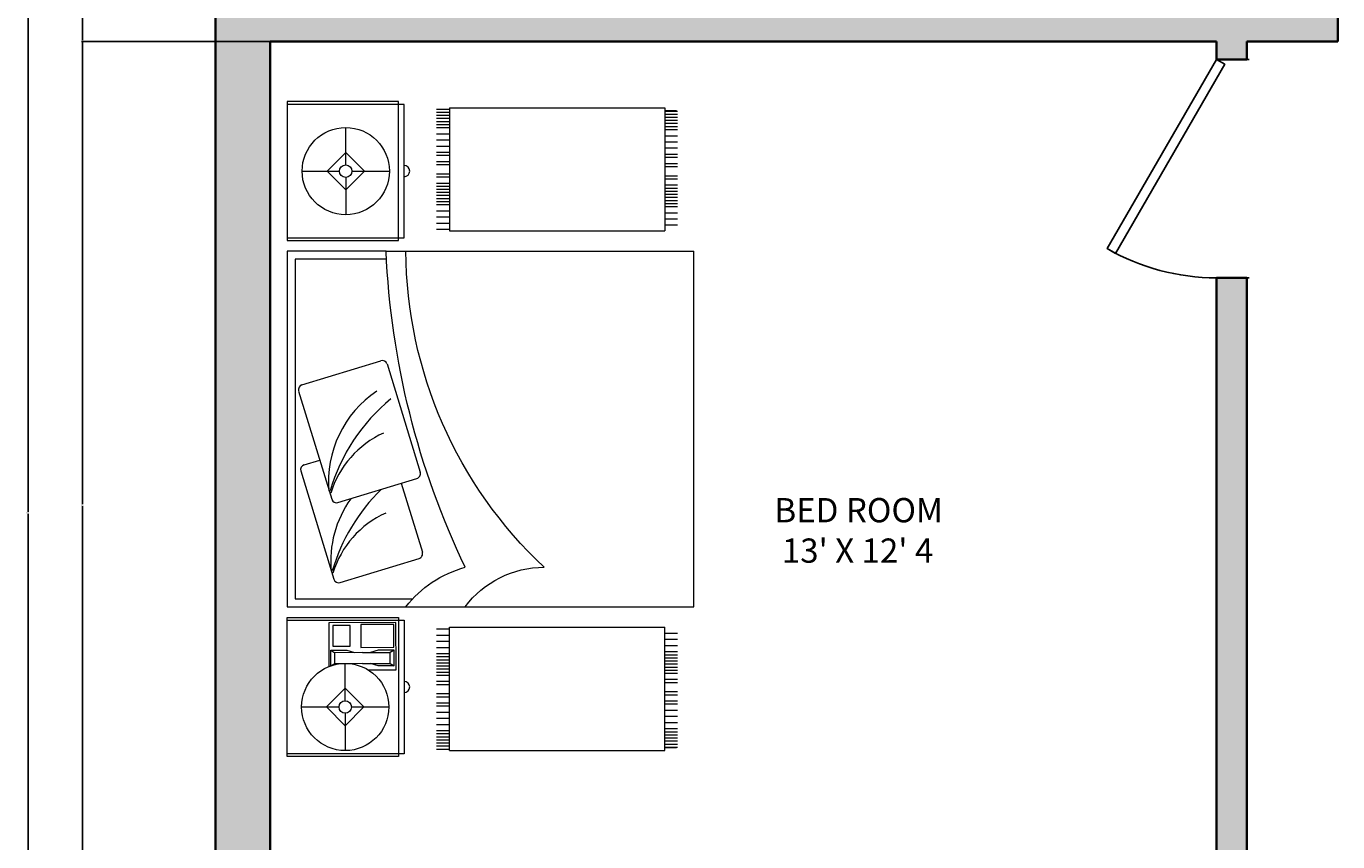
# Model space of a CAD drawing. Units: inches. Extents: x -30 to 437, y -29 to 647.
# Tile 7 of 15: x -30 to 187, y 255 to 389. Entities that reach past the tile are written whole.
import ezdxf

# ---------------------------------------------------------------- set-up
doc = ezdxf.new("R2010")
doc.units = ezdxf.units.IN
doc.header["$MEASUREMENT"] = 0
for name, color, linetype, lineweight in [('A-ANNO-DIMS', 2, 'Continuous', 18), ('A-AREA-IDEN', 7, 'Continuous', 18), ('A-WALL', 7, 'Continuous', 35), ('bedroom', 120, 'Continuous', 18), ('doors', 40, 'Continuous', 25)]:
    doc.layers.add(name, color=color, linetype=linetype, lineweight=lineweight)
doc.layers.add('A-WALL-PATT', color=251, linetype='Continuous', lineweight=13, true_color=0x636466)
doc.styles.get("Standard").update_dxf_attribs({"font": 'arial.ttf'})
doc.dimstyles.get("Standard").update_dxf_attribs({"dimtxt": 0.18, "dimasz": 0.18, "dimexe": 0.18, "dimexo": 0.0625, "dimgap": 0.09, "dimtad": 0, "dimtih": 1, "dimtoh": 1, "dimdec": 4, "dimzin": 0, "dimdsep": 46, "dimtxsty": 'Standard', "dimcen": 0.09, "dimadec": 0, "dimazin": 0, "dimtfac": 1, "dimtdec": 4, "dimtofl": 0, "dimtmove": 0, "dimatfit": 3, "dimfxl": 1, "dimtolj": 1, "dimtzin": 0, "dimarcsym": 0})

# ---------------------------------------------------------------- blocks, each defined once
blk = doc.blocks.new('3')
for p, q in [((185.8665, 224.6766), (185.8665, 225.2363)), ((185.8665, 225.2363), (186.566, 225.2363)), ((185.8805, 224.6487), (185.8805, 225.2363)), ((186.552, 225.2363), (186.552, 224.6487)), ((186.566, 225.2363), (186.566, 224.6766)), ((186.6199, 225.2363), (186.6199, 224.6399)), ((188.4089, 225.2363), (186.6199, 225.2363)), ((188.4089, 224.7393), (188.4089, 225.2363)), ((188.4627, 225.2363), (188.4627, 224.6766)), ((189.1623, 225.2363), (188.4627, 225.2363)), ((188.4767, 225.2363), (188.4767, 224.6486)), ((189.1483, 224.6486), (189.1483, 225.2363)), ((189.1623, 224.6766), (189.1623, 225.2363)), ((186.1157, 225.1643), (186.1157, 224.9763)), ((187.3034, 225.1683), (186.7581, 225.0015)), ((187.7059, 225.1793), (187.1607, 225.0124)), ((187.3344, 225.1518), (187.3586, 225.073)), ((187.737, 225.1628), (187.8585, 224.7657)), ((188.8125, 225.1618), (188.8125, 224.9738)), ((186.0216, 224.9449), (186.1157, 225.0389)), ((186.1157, 225.0389), (186.2097, 224.9449)), ((186.5397, 225.0274), (186.3193, 225.0266)), ((186.3215, 225.0167), (186.4008, 225.017)), ((186.3334, 224.9969), (186.3215, 225.0167)), ((186.3334, 224.9969), (186.389, 224.9971)), ((186.334, 224.858), (186.3334, 224.9969)), ((186.4008, 225.017), (186.389, 224.9971)), ((186.3895, 224.8582), (186.389, 224.9971)), ((186.4008, 225.017), (186.4011, 224.9376)), ((186.5409, 224.6901), (186.5397, 225.0274)), ((188.8125, 225.0365), (188.7185, 224.9424)), ((188.9065, 224.9424), (188.8125, 225.0365)), ((186.0843, 224.9449), (185.8963, 224.9449)), ((186.1157, 224.8509), (186.0216, 224.9449)), ((186.2097, 224.9449), (186.1157, 224.8509)), ((186.147, 224.9449), (186.335, 224.9449)), ((186.4011, 224.9376), (186.3894, 224.8979)), ((186.7416, 224.9704), (186.8631, 224.5734)), ((187.1442, 224.9814), (187.2657, 224.5843)), ((188.7812, 224.9424), (188.5931, 224.9424)), ((188.7185, 224.9424), (188.8125, 224.8484)), ((188.8125, 224.8484), (188.9065, 224.9424)), ((188.8438, 224.9424), (189.0319, 224.9424)), ((186.1157, 224.9136), (186.1157, 224.7256)), ((186.3314, 224.9055), (186.3338, 224.8977)), ((186.334, 224.858), (186.3345, 224.7191)), ((186.3895, 224.8582), (186.39, 224.7193)), ((188.8125, 224.9111), (188.8125, 224.723)), ((186.3023, 224.8297), (186.3029, 224.6892)), ((186.3224, 224.7786), (186.3341, 224.8183)), ((186.4017, 224.7789), (186.3897, 224.8185)), ((186.3227, 224.6992), (186.3224, 224.7786)), ((186.402, 224.6995), (186.4017, 224.7789)), ((187.842, 224.7347), (187.2967, 224.5678)), ((188.4089, 224.7393), (188.4089, 223.1907)), ((186.566, 224.6766), (185.8665, 224.6766)), ((186.3029, 224.6892), (186.5409, 224.6901)), ((186.3345, 224.7191), (186.3227, 224.6992)), ((186.3227, 224.6992), (186.402, 224.6995)), ((186.3345, 224.7191), (186.39, 224.7193)), ((186.402, 224.6995), (186.39, 224.7193)), ((187.2416, 224.6632), (186.8942, 224.5569)), ((188.4627, 224.6766), (189.1623, 224.6766)), ((186.552, 224.6487), (185.8805, 224.6487)), ((186.6199, 224.6399), (186.6199, 223.1907)), ((188.4767, 224.6486), (189.1483, 224.6486)), ((185.904, 224.4849, -0.9094), (185.904, 224.4204, -0.9094)), ((185.9195, 224.4849, -0.9094), (185.9195, 224.4204, -0.9094)), ((185.9195, 224.4849, -0.9094), (185.9195, 224.4204, -0.9094)), ((185.935, 224.4849, -0.9094), (185.935, 224.4204, -0.9094)), ((185.9505, 224.4849, -0.9094), (185.9505, 224.4204, -0.9094)), ((185.966, 224.4849, -0.9094), (185.966, 224.4204, -0.9094)), ((185.9815, 224.4849, -0.9094), (185.9815, 224.4204, -0.9094)), ((185.997, 224.4849, -0.9094), (185.997, 224.4204, -0.9094)), ((186.028, 224.4849, -0.9094), (186.028, 224.4204, -0.9094)), ((186.059, 224.4849, -0.9094), (186.059, 224.4204, -0.9094)), ((186.09, 224.4849, -0.9094), (186.09, 224.4204, -0.9094)), ((186.09, 224.4849, -0.9094), (186.09, 224.4204, -0.9094)), ((186.121, 224.4849, -0.9094), (186.121, 224.4204, -0.9094)), ((186.1365, 224.4849, -0.9094), (186.1365, 224.4204, -0.9094)), ((186.1675, 224.4849, -0.9094), (186.1675, 224.4204, -0.9094)), ((186.183, 224.4849, -0.9094), (186.183, 224.4204, -0.9094)), ((186.2295, 224.4849, -0.9094), (186.2295, 224.4204, -0.9094)), ((186.245, 224.4849, -0.9094), (186.245, 224.4204, -0.9094)), ((186.276, 224.4849, -0.9094), (186.276, 224.4204, -0.9094)), ((186.2915, 224.4849, -0.9094), (186.2915, 224.4204, -0.9094)), ((186.307, 224.4849, -0.9094), (186.307, 224.4204, -0.9094)), ((186.3225, 224.4849, -0.9094), (186.3225, 224.4204, -0.9094)), ((186.338, 224.4849, -0.9094), (186.338, 224.4204, -0.9094)), ((186.3535, 224.4849, -0.9094), (186.3535, 224.4204, -0.9094)), ((186.369, 224.4849, -0.9094), (186.369, 224.4204, -0.9094)), ((186.3845, 224.4849, -0.9094), (186.3845, 224.4204, -0.9094)), ((186.4155, 224.4849, -0.9094), (186.4155, 224.4204, -0.9094)), ((186.4465, 224.4849, -0.9094), (186.4465, 224.4204, -0.9094)), ((186.4775, 224.4849, -0.9094), (186.4775, 224.4204, -0.9094)), ((186.5085, 224.4849, -0.9094), (186.5085, 224.4204, -0.9094)), ((188.5202, 224.4849, -0.9094), (188.5202, 224.4204, -0.9094)), ((188.5512, 224.4849, -0.9094), (188.5512, 224.4204, -0.9094)), ((188.5822, 224.4849, -0.9094), (188.5822, 224.4204, -0.9094)), ((188.6132, 224.4849, -0.9094), (188.6132, 224.4204, -0.9094)), ((188.6442, 224.4849, -0.9094), (188.6442, 224.4204, -0.9094)), ((188.6597, 224.4849, -0.9094), (188.6597, 224.4204, -0.9094)), ((188.6752, 224.4849, -0.9094), (188.6752, 224.4204, -0.9094)), ((188.6907, 224.4849, -0.9094), (188.6907, 224.4204, -0.9094)), ((188.7062, 224.4849, -0.9094), (188.7062, 224.4204, -0.9094)), ((188.7217, 224.4849, -0.9094), (188.7217, 224.4204, -0.9094)), ((188.7372, 224.4849, -0.9094), (188.7372, 224.4204, -0.9094)), ((188.7527, 224.4849, -0.9094), (188.7527, 224.4204, -0.9094)), ((188.7837, 224.4849, -0.9094), (188.7837, 224.4204, -0.9094)), ((188.7992, 224.4849, -0.9094), (188.7992, 224.4204, -0.9094)), ((188.8457, 224.4849, -0.9094), (188.8457, 224.4204, -0.9094)), ((188.8612, 224.4849, -0.9094), (188.8612, 224.4204, -0.9094)), ((188.8922, 224.4849, -0.9094), (188.8922, 224.4204, -0.9094)), ((188.9077, 224.4849, -0.9094), (188.9077, 224.4204, -0.9094)), ((188.9387, 224.4849, -0.9094), (188.9387, 224.4204, -0.9094)), ((188.9387, 224.4849, -0.9094), (188.9387, 224.4204, -0.9094)), ((188.9697, 224.4849, -0.9094), (188.9697, 224.4204, -0.9094)), ((189.0007, 224.4849, -0.9094), (189.0007, 224.4204, -0.9094)), ((189.0317, 224.4849, -0.9094), (189.0317, 224.4204, -0.9094)), ((189.0472, 224.4849, -0.9094), (189.0472, 224.4204, -0.9094)), ((189.0627, 224.4849, -0.9094), (189.0627, 224.4204, -0.9094)), ((189.0782, 224.4849, -0.9094), (189.0782, 224.4204, -0.9094)), ((189.0937, 224.4849, -0.9094), (189.0937, 224.4204, -0.9094)), ((189.1092, 224.4849, -0.9094), (189.1092, 224.4204, -0.9094)), ((189.1092, 224.4849, -0.9094), (189.1092, 224.4204, -0.9094)), ((189.1247, 224.4849, -0.9094), (189.1247, 224.4204, -0.9094)), ((185.8974, 224.4204, -0.9094), (185.8974, 223.3378, -0.9094)), ((185.8974, 224.4204, -0.9094), (186.5174, 224.4204, -0.9094)), ((186.5174, 224.4204, -0.9094), (186.5174, 223.3378, -0.9094)), ((189.1313, 224.4204, -0.9094), (188.5113, 224.4204, -0.9094)), ((188.5113, 224.4204, -0.9094), (188.5113, 223.3378, -0.9094)), ((189.1313, 224.4204, -0.9094), (189.1313, 223.3378, -0.9094)), ((185.8974, 223.3378, -0.9094), (186.5174, 223.3378, -0.9094)), ((185.9114, 223.3378, -0.9094), (185.9114, 223.2789, -0.9094)), ((185.9114, 223.3378, -0.9094), (185.9114, 223.2789, -0.9094)), ((185.9114, 223.3378, -0.9094), (185.9114, 223.2789, -0.9094)), ((185.9138, 223.3378, -0.9094), (185.9138, 223.2732, -0.9094)), ((185.9293, 223.3378, -0.9094), (185.9293, 223.2732, -0.9094)), ((185.9293, 223.3378, -0.9094), (185.9293, 223.2732, -0.9094)), ((185.9448, 223.3378, -0.9094), (185.9448, 223.2732, -0.9094)), ((185.9603, 223.3378, -0.9094), (185.9603, 223.2732, -0.9094)), ((185.9758, 223.3378, -0.9094), (185.9758, 223.2732, -0.9094)), ((185.9913, 223.3378, -0.9094), (185.9913, 223.2732, -0.9094)), ((186.0068, 223.3378, -0.9094), (186.0068, 223.2732, -0.9094)), ((186.0378, 223.3378, -0.9094), (186.0378, 223.2732, -0.9094)), ((186.0688, 223.3378, -0.9094), (186.0688, 223.2732, -0.9094)), ((186.0998, 223.3378, -0.9094), (186.0998, 223.2732, -0.9094)), ((186.0998, 223.3378, -0.9094), (186.0998, 223.2732, -0.9094)), ((186.1308, 223.3378, -0.9094), (186.1308, 223.2732, -0.9094)), ((186.1463, 223.3378, -0.9094), (186.1463, 223.2732, -0.9094)), ((186.1773, 223.3378, -0.9094), (186.1773, 223.2732, -0.9094)), ((186.1928, 223.3378, -0.9094), (186.1928, 223.2732, -0.9094)), ((186.2393, 223.3378, -0.9094), (186.2393, 223.2732, -0.9094)), ((186.2548, 223.3378, -0.9094), (186.2548, 223.2732, -0.9094)), ((186.2858, 223.3378, -0.9094), (186.2858, 223.2732, -0.9094)), ((186.3013, 223.3378, -0.9094), (186.3013, 223.2732, -0.9094)), ((186.3168, 223.3378, -0.9094), (186.3168, 223.2732, -0.9094)), ((186.3323, 223.3378, -0.9094), (186.3323, 223.2732, -0.9094)), ((186.3478, 223.3378, -0.9094), (186.3478, 223.2732, -0.9094)), ((186.3633, 223.3378, -0.9094), (186.3633, 223.2732, -0.9094)), ((186.3788, 223.3378, -0.9094), (186.3788, 223.2732, -0.9094)), ((186.3943, 223.3378, -0.9094), (186.3943, 223.2732, -0.9094)), ((186.4253, 223.3378, -0.9094), (186.4253, 223.2732, -0.9094)), ((186.4563, 223.3378, -0.9094), (186.4563, 223.2732, -0.9094)), ((186.4873, 223.3378, -0.9094), (186.4873, 223.2732, -0.9094)), ((189.1313, 223.3378, -0.9094), (188.5113, 223.3378, -0.9094)), ((188.5414, 223.3378, -0.9094), (188.5414, 223.2732, -0.9094)), ((188.5724, 223.3378, -0.9094), (188.5724, 223.2732, -0.9094)), ((188.6034, 223.3378, -0.9094), (188.6034, 223.2732, -0.9094)), ((188.6344, 223.3378, -0.9094), (188.6344, 223.2732, -0.9094)), ((188.6499, 223.3378, -0.9094), (188.6499, 223.2732, -0.9094)), ((188.6654, 223.3378, -0.9094), (188.6654, 223.2732, -0.9094)), ((188.6809, 223.3378, -0.9094), (188.6809, 223.2732, -0.9094)), ((188.6964, 223.3378, -0.9094), (188.6964, 223.2732, -0.9094)), ((188.7119, 223.3378, -0.9094), (188.7119, 223.2732, -0.9094)), ((188.7274, 223.3378, -0.9094), (188.7274, 223.2732, -0.9094)), ((188.7429, 223.3378, -0.9094), (188.7429, 223.2732, -0.9094)), ((188.7739, 223.3378, -0.9094), (188.7739, 223.2732, -0.9094)), ((188.7894, 223.3378, -0.9094), (188.7894, 223.2732, -0.9094)), ((188.8359, 223.3378, -0.9094), (188.8359, 223.2732, -0.9094)), ((188.8514, 223.3378, -0.9094), (188.8514, 223.2732, -0.9094)), ((188.8824, 223.3378, -0.9094), (188.8824, 223.2732, -0.9094)), ((188.8979, 223.3378, -0.9094), (188.8979, 223.2732, -0.9094)), ((188.9289, 223.3378, -0.9094), (188.9289, 223.2732, -0.9094)), ((188.9289, 223.3378, -0.9094), (188.9289, 223.2732, -0.9094)), ((188.9599, 223.3378, -0.9094), (188.9599, 223.2732, -0.9094)), ((188.9909, 223.3378, -0.9094), (188.9909, 223.2732, -0.9094)), ((189.022, 223.3378, -0.9094), (189.022, 223.2732, -0.9094)), ((189.0375, 223.3378, -0.9094), (189.0375, 223.2732, -0.9094)), ((189.053, 223.3378, -0.9094), (189.053, 223.2732, -0.9094)), ((189.0685, 223.3378, -0.9094), (189.0685, 223.2732, -0.9094)), ((189.084, 223.3378, -0.9094), (189.084, 223.2732, -0.9094)), ((189.0995, 223.3378, -0.9094), (189.0995, 223.2732, -0.9094)), ((189.0995, 223.3378, -0.9094), (189.0995, 223.2732, -0.9094)), ((189.115, 223.3378, -0.9094), (189.115, 223.2732, -0.9094)), ((189.1173, 223.3378, -0.9094), (189.1173, 223.2789, -0.9094)), ((189.1173, 223.3378, -0.9094), (189.1173, 223.2789, -0.9094)), ((189.1173, 223.3378, -0.9094), (189.1173, 223.2789, -0.9094)), ((186.6199, 223.1907), (188.4089, 223.1907))]:
    blk.add_line(p, q)
blk.add_lwpolyline([(188.3691, 224.7374), (188.3691, 225.1965), (186.6596, 225.1965), (186.6596, 224.606)])
for points in [[(186.4217, 225.0072), (186.422, 224.9199), (186.5252, 224.9202), (186.5249, 225.0075)], [(186.4153, 224.8663), (186.4159, 224.6996), (186.531, 224.7), (186.5304, 224.8667)]]:
    blk.add_lwpolyline(points, close=True)
for points in [[(186.6199, 224.6399, -0.162278), (186.8186, 224.3418, -0.100664), (188.4089, 224.7393, -0.100664)], [(186.6199, 224.3418, -0.236068), (186.8186, 223.9442, -0.205258), (188.4089, 224.6399, -0.205258)]]:
    blk.add_lwpolyline(points, format="xyb")
for centre, radius in [((186.1157, 224.9449), 0.2194), ((188.8125, 224.9424), 0.2194), ((186.1157, 224.9449), 0.0313), ((188.8125, 224.9424), 0.0313)]:
    blk.add_circle(centre, radius)
for centre, radius, start, end in [((187.3107, 225.1446), 0.0248, 17.0142, 107.0142), ((187.7132, 225.1555), 0.0248, 17.0142, 107.0142), ((186.7654, 224.9777), 0.0248, 107.0142, 197.0142), ((186.6474, 224.5408), 0.4873, 24.22087, 73.06906), ((186.8477, 224.4712), 0.5468, 54.68511, 95.16051), ((186.5359, 224.1054), 0.9426, 44.27274, 73.71889), ((187.1679, 224.9887), 0.0248, 107.0142, 197.0142), ((187.0499, 224.5517), 0.4873, 24.22087, 73.06906), ((187.2502, 224.4821), 0.5468, 33.78007, 95.16051), ((186.9385, 224.1164), 0.9426, 39.40233, 73.71889), ((187.8347, 224.7585), 0.0248, 287.0142, 17.0142), ((186.2163, 224.6487), 0.028, 180, 0), ((188.8125, 224.6486), 0.028, 180, 0), ((186.8869, 224.5806), 0.0248, 197.0142, 287.0142), ((187.2894, 224.5916), 0.0248, 197.0142, 287.0142)]:
    blk.add_arc(centre, radius, start, end)
blk = doc.blocks.new('*U7')
for p, q in [((0, 0), (0, 6)), ((40, 0), (40, 6))]:
    blk.add_line(p, q)
blk.add_lwpolyline([(0, 0), (34.64, -20), (35.52, -18.48), (0.87, 1.52)], close=True)
blk.add_arc((0, 0), 40, 330, 0)
blk = doc.blocks.new('*D26')
at = {"layer": 'A-ANNO-DIMS', "color": 0, "lineweight": -2, "transparency": 16777216}
for p, q in [((1.61, 615.55), (-29.41, 615.55)), ((-29.23, 615.37), (-29.23, 308.98)), ((-29.23, 2.23), (-29.23, 308.62)), ((1.61, 2.05), (-29.41, 2.05))]:
    blk.add_line(p, q, dxfattribs=at)
at = {"layer": 'A-ANNO-DIMS', "color": 0, "transparency": 16777216}
for points in [[(-29.26, 615.37), (-29.2, 615.37), (-29.23, 615.55)], [(-29.26, 2.23), (-29.2, 2.23), (-29.23, 2.05)]]:
    blk.add_solid(points, dxfattribs=at)
at = {"layer": 'Defpoints', "color": 0, "transparency": 16777216}
for p in [(-29.23, 615.55), (1.67, 615.55), (1.67, 2.05)]:
    blk.add_point(p, dxfattribs=at)
at = {"layer": 'A-ANNO-DIMS', "color": 0, "transparency": 16777216, "insert": (-29.23, 308.8), "char_height": 0.18, "attachment_point": 5}
blk.add_mtext('\\A1;613.5', dxfattribs=at)
blk = doc.blocks.new('*D32')
at = {"layer": 'A-ANNO-DIMS', "color": 0, "lineweight": -2, "transparency": 16777216}
for p, q in [((10.61, 386.55), (-20.41, 386.55)), ((-20.23, 386.37), (-20.23, 310.23)), ((-20.23, 233.73), (-20.23, 309.87)), ((10.61, 233.55), (-20.41, 233.55))]:
    blk.add_line(p, q, dxfattribs=at)
at = {"layer": 'A-ANNO-DIMS', "color": 0, "transparency": 16777216}
for points in [[(-20.26, 386.37), (-20.2, 386.37), (-20.23, 386.55)], [(-20.26, 233.73), (-20.2, 233.73), (-20.23, 233.55)]]:
    blk.add_solid(points, dxfattribs=at)
at = {"layer": 'Defpoints', "color": 0, "transparency": 16777216}
for p in [(-20.23, 386.55), (10.67, 386.55), (10.67, 233.55)]:
    blk.add_point(p, dxfattribs=at)
at = {"layer": 'A-ANNO-DIMS', "color": 0, "transparency": 16777216, "insert": (-20.23, 310.05), "char_height": 0.18, "attachment_point": 5}
blk.add_mtext('\\A1;153', dxfattribs=at)
blk = doc.blocks.new('*D33')
at = {"layer": 'A-ANNO-DIMS', "color": 0, "lineweight": -2, "transparency": 16777216}
for p, q in [((10.61, 547.55), (-20.41, 547.55)), ((-20.23, 547.37), (-20.23, 467.23)), ((-20.23, 386.73), (-20.23, 466.87)), ((10.61, 386.55), (-20.41, 386.55))]:
    blk.add_line(p, q, dxfattribs=at)
at = {"layer": 'A-ANNO-DIMS', "color": 0, "transparency": 16777216}
for points in [[(-20.26, 547.37), (-20.2, 547.37), (-20.23, 547.55)], [(-20.26, 386.73), (-20.2, 386.73), (-20.23, 386.55)]]:
    blk.add_solid(points, dxfattribs=at)
at = {"layer": 'Defpoints', "color": 0, "transparency": 16777216}
for p in [(-20.23, 547.55), (10.67, 547.55), (10.67, 386.55)]:
    blk.add_point(p, dxfattribs=at)
at = {"layer": 'A-ANNO-DIMS', "color": 0, "transparency": 16777216, "insert": (-20.23, 467.05), "char_height": 0.18, "attachment_point": 5}
blk.add_mtext('\\A1;161', dxfattribs=at)

msp = doc.modelspace()

# ---------------------------------------------------------------- hatches: boundary and pattern name
at = {"layer": 'A-WALL-PATT'}
h = msp.add_hatch(color=256, dxfattribs=at)
h.dxf.hatch_style = 1
h.paths.add_polyline_path([(393.6054, 183.2352), (369.6054, 183.2352), (369.6054, 213.2352), (393.6054, 213.2352), (393.6054, 207.2352), (394.6054, 207.2352), (394.6054, 211.2352), (395.6054, 211.2352), (395.6054, 185.2352), (394.6054, 185.2352), (394.6054, 189.2352), (393.6054, 189.2352)], flags=0)
h.paths.add_polyline_path([(384.6054, 189.2352, -1), (390.6054, 189.2352, -1)], flags=0)
h.paths.add_polyline_path([(385.6054, 189.2352, -1), (389.6054, 189.2352, -1)], flags=0)
h.paths.add_polyline_path([(374.6054, 189.2352, -1), (382.6054, 189.2352, -1)], flags=0)
h.paths.add_polyline_path([(386.6054, 189.2352, -1), (388.6054, 189.2352, -1)], flags=0)
h.paths.add_polyline_path([(375.6054, 189.2352, -1), (381.6054, 189.2352, -1)], flags=0)
h.paths.add_polyline_path([(376.6054, 189.2352, -1), (380.6054, 189.2352, -1)], flags=0)
h.paths.add_polyline_path([(377.6054, 189.2352, -1), (379.6054, 189.2352, -1)], flags=0)
h.paths.add_polyline_path([(390.6054, 195.2352), (374.6054, 195.2352), (374.6054, 201.2352), (390.6054, 201.2352)], flags=0)
h.paths.add_polyline_path([(389.6054, 196.2352), (375.6054, 196.2352), (375.6054, 200.2352), (389.6054, 200.2352)], flags=0)
h.paths.add_polyline_path([(383.6054, 207.2352, -1), (391.6054, 207.2352, -1)], flags=0)
h.paths.add_polyline_path([(384.6054, 207.2352, -1), (390.6054, 207.2352, -1)], flags=0)
h.paths.add_polyline_path([(385.6054, 207.2352, -1), (389.6054, 207.2352, -1)], flags=0)
h.paths.add_polyline_path([(386.6054, 207.2352, -1), (388.6054, 207.2352, -1)], flags=0)
h.paths.add_polyline_path([(375.6054, 207.2352, -1), (381.6054, 207.2352, -1)], flags=0)
h.paths.add_polyline_path([(376.6054, 207.2352, -1), (380.6054, 207.2352, -1)], flags=0)
h.paths.add_polyline_path([(377.6054, 207.2352, -1), (379.6054, 207.2352, -1)], flags=0)
h.paths.add_polyline_path([(305.5437, 160.3663, -0.41421356), (304.0437, 158.8663), (271.0437, 158.8663, -0.41421356), (269.5437, 160.3663), (269.5437, 178.3663, -0.41421356), (271.0437, 179.8663), (304.0437, 179.8663, -0.41421356), (305.5437, 178.3663)], flags=0)
h.paths.add_polyline_path([(304.0437, 165.3663, -0.41421356), (303.0437, 164.3663), (289.2937, 164.3663, -0.41421356), (288.2937, 165.3663), (288.2937, 177.3663, -0.41421356), (289.2937, 178.3663), (303.0437, 178.3663, -0.41421356), (304.0437, 177.3663)], flags=0)
h.paths.add_polyline_path([(296.5437, 171.3663, -1), (295.5437, 171.3663, -1)], flags=0)
h.paths.add_polyline_path([(286.7937, 165.3663, -0.41421356), (285.7937, 164.3663), (272.0437, 164.3663, -0.41421356), (271.0437, 165.3663), (271.0437, 177.3663, -0.41421356), (272.0437, 178.3663), (285.7937, 178.3663, -0.41421356), (286.7937, 177.3663)], flags=0)
h.paths.add_polyline_path([(279.5437, 171.3663, -1), (278.5437, 171.3663, -1)], flags=0)
h.paths.add_polyline_path([(360.6737, 290.5474), (360.6737, 300.5474), (396.6737, 300.5474), (396.6737, 290.5474)], flags=0)
h.paths.add_polyline_path([(259.6737, 124.5474), (259.6737, 114.5474), (171.6737, 114.5474), (171.6737, 124.5474)], flags=0)
h.paths.add_polyline_path([(288.0737, 215.3705), (286.7097, 214.583), (268.7097, 245.7599), (270.0737, 246.5474)], flags=0)
h.paths.add_polyline_path([(259.6737, 168.5474), (256.6737, 168.5474), (256.6737, 173.5474), (256.6737, 179.0224), (255.8753, 177.6395), (224.2956, 195.872, 0.12053744), (220.1737, 179.0224, 0.12053744), (216.0518, 195.872), (184.4721, 177.6395), (183.6737, 179.0224), (215.2836, 197.2724), (216.0821, 195.8895), (216.0518, 195.872, -0.12053744), (220.1737, 179.0224, -0.12053744), (224.2956, 195.872), (224.2653, 195.8895), (225.0638, 197.2724), (256.6737, 179.0224), (256.6737, 173.5474), (259.6737, 173.5474)], flags=0)
h.paths.add_polyline_path([(386.7943, 325.4601), (372.6871, 325.4601), (372.6871, 339.5673), (386.7943, 339.5673)], flags=0)
h.paths.add_polyline_path([(359.5875, 343.7429), (357.7905, 343.7429), (357.7905, 327.9179), (359.3933, 327.9179, 0.41420885), (361.5302, 330.0549), (361.5302, 341.8434, 0.41436161)], flags=0)
h.paths.add_polyline_path([(341.7887, 323.1235, -0.11921667), (340.7839, 323.1235)], flags=0)
h.paths.add_polyline_path([(379.6332, 328.8632), (379.6332, 332.2699), (376.0992, 332.2699, 0.39427733)], flags=0)
h.paths.add_polyline_path([(375.5299, 332.459, -1), (383.8511, 332.459, -1)], flags=0)
h.paths.add_polyline_path([(388.9363, 344.7425), (372.5309, 344.7425, -0.41421356), (370.394, 346.8794), (370.394, 347.5594, -0.39085173), (372.3472, 349.7005, -0.43951011), (370.394, 351.4933), (370.394, 365.1894, -0.40305452), (372.2191, 367.1298, -0.41839453), (370.394, 368.9291), (370.394, 382.6251, -0.40885826), (372.2519, 384.5722, -0.42377324), (370.394, 386.3707), (370.394, 400.0667, -0.38660687), (372.1327, 402.0094), (372.531, 402.0094, -0.41421834), (370.394, 404.1464), (370.394, 404.7778, -0.41420891), (372.5309, 406.9147), (388.9363, 406.9147, -0.41421821), (391.0733, 404.7778), (391.0733, 346.8794, -0.41421356)], flags=0)
edge = h.paths.add_edge_path(flags=0)
edge.add_spline(control_points=[(349.3585, 363.204), (349.0859, 363.204), (348.8133, 363.2227), (348.2712, 363.2973), (348.0016, 363.3531), (347.3533, 363.5328), (346.9776, 363.6755), (346.2445, 364.0308), (345.887, 364.2432), (345.1953, 364.7329), (344.8611, 365.0101), (344.2197, 365.6237), (343.9125, 365.9603), (343.211, 366.8336), (342.8313, 367.3965), (342.1401, 368.6117), (341.8286, 369.2641), (341.2807, 370.64), (341.0443, 371.3636), (340.6522, 372.8619), (340.4964, 373.6367), (340.2695, 375.2158), (340.1983, 376.0203), (340.142, 377.6365), (340.157, 378.4483), (340.2729, 380.0567), (340.3738, 380.8533), (340.6589, 382.4093), (340.8432, 383.1686), (341.2906, 384.629), (341.5538, 385.3301), (342.1531, 386.6544), (342.4891, 387.2776), (343.2266, 388.4288), (343.6281, 388.9567), (344.4879, 389.9012), (344.9463, 390.3178), (345.7981, 390.9428), (346.182, 391.1771), (346.9712, 391.5648), (347.3766, 391.7182), (348.2004, 391.9387), (348.6189, 392.0058), (349.4588, 392.0508), (349.8801, 392.0288), (350.7146, 391.8966), (351.1278, 391.7865), (351.9366, 391.4822), (352.3323, 391.2882), (353.0989, 390.8223), (353.4699, 390.5504), (354.1819, 389.9355), (354.5229, 389.5924), (355.1706, 388.8418), (355.4772, 388.4343), (356.1315, 387.4422), (356.4671, 386.8397), (357.0692, 385.5581), (357.3356, 384.879), (357.7933, 383.4624), (357.9846, 382.725), (358.2875, 381.2112), (358.3992, 380.4349), (358.5404, 378.8643), (358.5699, 378.0699), (358.546, 376.4841), (358.4926, 375.6928), (358.3042, 374.1343), (358.1692, 373.3672), (357.8207, 371.8774), (357.6072, 371.1549), (357.1067, 369.7735), (356.8196, 369.1148), (356.1782, 367.8787), (355.8238, 367.3013), (355.0551, 366.244), (354.6408, 365.7641), (353.7607, 364.9161), (353.2948, 364.5481), (352.445, 364.0149), (352.0701, 363.822), (351.3034, 363.5117), (350.9116, 363.3943), (350.1325, 363.2418), (349.7455, 363.204), (349.3585, 363.204)], knot_values=[3.14159265, 3.14159265, 3.14159265, 3.14159265, 3.22691715, 3.22691715, 3.31224165, 3.31224165, 3.43426671, 3.43426671, 3.55629177, 3.55629177, 3.67831683, 3.67831683, 3.8003419, 3.8003419, 3.97157384, 3.97157384, 4.14280577, 4.14280577, 4.31403771, 4.31403771, 4.48526965, 4.48526965, 4.65650159, 4.65650159, 4.82773353, 4.82773353, 4.99896547, 4.99896547, 5.1701974, 5.1701974, 5.34142934, 5.34142934, 5.51266128, 5.51266128, 5.68389322, 5.68389322, 5.85512516, 5.85512516, 5.98669107, 5.98669107, 6.11825699, 6.11825699, 6.24982291, 6.24982291, 6.38138882, 6.38138882, 6.51295474, 6.51295474, 6.64452065, 6.64452065, 6.77608657, 6.77608657, 6.90765249, 6.90765249, 7.0392184, 7.0392184, 7.20701563, 7.20701563, 7.37481286, 7.37481286, 7.54261009, 7.54261009, 7.71040732, 7.71040732, 7.87820455, 7.87820455, 8.04600178, 8.04600178, 8.21379901, 8.21379901, 8.38159624, 8.38159624, 8.54939347, 8.54939347, 8.7171907, 8.7171907, 8.88498794, 8.88498794, 9.05278517, 9.05278517, 9.17820699, 9.17820699, 9.30362881, 9.30362881, 9.42477796, 9.42477796, 9.42477796, 9.42477796], degree=3, periodic=0)
edge.add_line((341.1696, 384.3006), (341.2012, 384.2808))
edge = h.paths.add_edge_path(flags=0)
edge.add_line((344.3353, 388.7801), (344.317, 388.7915))
edge.add_ellipse((349.3585, 377.6204), major_axis=(0, -13.7895), ratio=0.62186025, start_angle=-244.867444, end_angle=-124.769923)
h.paths.add_polyline_path([(163.6737, 163.1474), (132.4968, 145.1474), (131.7093, 146.5114), (162.8862, 164.5114)], flags=0)
h.paths.add_polyline_path([(366.4355, 409.0896, -0.41423669), (364.2985, 406.9525, -0.4913499), (361.5302, 408.8973), (361.5302, 420.6405, 0.41421356), (359.3932, 422.7775), (357.7905, 422.7775), (357.7905, 406.9525), (359.6317, 406.9525, 0.42741026), (361.5332, 408.9757, 0.39869469), (363.6672, 406.9525, 0.51958103), (366.4355, 409.0895)], flags=0)
h.paths.add_polyline_path([(386.7943, 410.9671), (372.6871, 410.9671), (372.6871, 425.0742), (386.7943, 425.0742)], flags=0)
h.paths.add_polyline_path([(379.6332, 414.3701), (379.6332, 417.7768), (376.0992, 417.7768, 0.39427733)], flags=0)
h.paths.add_polyline_path([(375.5299, 417.966, -1), (383.8511, 417.966, -1)], flags=0)
h.paths.add_polyline_path([(150.0377, 351.583), (148.6737, 352.3705), (166.6737, 383.5474), (168.0377, 382.7599)], flags=0)
h.paths.add_polyline_path([(91.6737, 234.1974), (66.559, 219.6974), (65.9246, 220.7962), (91.0393, 235.2962)], flags=0)
h.paths.add_polyline_path([(255.4612, 443.5834), (254.6737, 444.9474), (285.8506, 462.9474), (286.6381, 461.5834)], flags=0)
h.paths.add_polyline_path([(176.2737, 394.5474), (158.2737, 425.7243), (159.6377, 426.5118), (177.6377, 395.3349)], flags=0)
h.paths.add_polyline_path([(243.6737, 439.5474), (243.0393, 438.4486), (217.9246, 452.9486), (218.559, 454.0474)], flags=0)
h.paths.add_polyline_path([(38.1264, 269.8429), (40.2408, 269.8429), (40.2408, 270.3508), (38.1264, 270.3508)], flags=0)
h.paths.add_polyline_path([(75.7157, 289.9439), (40.2408, 289.9439), (38.1264, 289.6524), (40.2408, 289.6524)], flags=0)
h.paths.add_polyline_path([(75.7157, 270.0846), (77.6447, 270.0846), (77.6697, 270.1626), (75.7175, 270.1626)], flags=0)
h.paths.add_polyline_path([(80.5373, 293.3002), (33.0467, 293.3002), (13.5054, 293.3002), (13.5054, 351.9244), (29.7898, 351.9244), (80.5373, 351.9244)], flags=0)
h.paths.add_polyline_path([(46.0261, 212.466, -0.50131678), (27.1651, 207.5106), (21.165, 209.5107), (21.165, 206.5107), (22.665, 206.5107), (22.665, 203.5107), (21.165, 203.5107), (21.165, 203.0107), (13.165, 203.0107), (13.165, 224.0107), (21.165, 224.0107), (21.165, 217.5107), (27.1649, 219.5106, -0.50132349), (46.0261, 214.5554, -0.13289091)], flags=0)
h.paths.add_polyline_path([(44.688, 211.8666, -0.48007965), (27.165, 209.5107), (27.165, 217.5107, -0.4800795), (44.688, 215.1547, -0.21500378)], flags=0)
h.paths.add_polyline_path([(19.415, 204.0107), (15.165, 204.0107, -0.41421356), (14.165, 204.7607), (14.165, 222.0107, -0.41421356), (14.915, 223.0107), (19.165, 223.0107, -0.41421356), (20.165, 222.2607), (20.165, 205.0107, -0.41421356)], flags=0)
h.paths.add_polyline_path([(32.7608, 269.0719), (31.8439, 269.0719), (31.8439, 268.6134), (13.5054, 268.6134), (13.5054, 291.5366), (31.8439, 291.5366), (32.7608, 291.0781), (32.7608, 280.9919, -1), (32.7608, 279.1581)], flags=0)
h.paths.add_polyline_path([(40.2408, 360.1436), (38.1264, 360.1436), (38.1264, 359.6357), (40.2408, 359.6357)], flags=0)
h.paths.add_polyline_path([(75.7157, 355.2807), (40.2408, 355.2807), (38.1264, 355.5722), (40.2408, 355.5722), (40.2408, 355.2807), (75.7157, 355.2807), (75.7157, 375.5982), (40.2408, 375.5982), (38.1264, 375.3817), (40.2408, 375.3817), (40.2408, 375.5982), (75.7157, 375.5982), (77.9733, 375.062), (75.7175, 375.062), (75.7175, 374.554)], flags=0)
h.paths.add_polyline_path([(42.8174, 299.814, 0.13867074), (34.1602, 294.603), (14.8081, 294.603), (14.8081, 350.6216), (29.8539, 350.6216, 0.09822056)], flags=0)
h.paths.add_polyline_path([(15.8636, 276.7781, -0.30640166), (20.3757, 283.4499), (20.3483, 290.6726), (31.4014, 290.7146), (31.4309, 282.9124), (26.8287, 282.895, -0.26006276), (30.241, 276.7781, -1)], flags=0)
h.paths.add_polyline_path([(26.1332, 276.7781), (23.0523, 273.6972), (19.9714, 276.7781), (23.0523, 279.8589), (23.0523, 283.9209), (21.3493, 283.9145), (20.7006, 283.5219), (20.6907, 286.1226), (23.2914, 286.1325), (25.8936, 285.7522), (27.1939, 285.7572), (28.4928, 286.1522), (31.0935, 286.1621), (31.0918, 286.6172), (25.6303, 286.5965), (25.616, 290.3675), (31.0775, 290.3882), (31.0918, 286.6172), (31.1034, 283.5614), (28.5027, 283.5515), (25.9005, 283.9317), (23.0523, 283.9209), (23.0523, 279.8589)], flags=0)
h.paths.add_polyline_path([(24.0793, 276.7781, -1), (22.0253, 276.7781, -1)], flags=0)
h.paths.add_polyline_path([(35.7687, 302.2895, -0.41421356), (35.2283, 301.2726), (22.2164, 297.2909, -0.41421356), (21.1995, 297.8313), (15.7317, 315.6996, -0.41421356), (16.2721, 316.7165), (18.8554, 317.507), (15.3721, 328.8904, -0.41421356), (15.9125, 329.9073), (28.9244, 333.889, -0.41421356), (29.9414, 333.3486), (35.4091, 315.4802, -0.41421356), (34.8687, 314.4633), (32.2854, 313.6728)], flags=0)
h.paths.add_polyline_path([(361.3728, 532.6207), (302.7487, 532.6207), (302.7487, 580.1113), (302.7487, 599.6527), (361.3728, 599.6527), (361.3728, 583.3682)], flags=0)
h.paths.add_polyline_path([(370.1, 575.0316), (370.1, 572.9172), (370.6079, 572.9172), (370.6079, 575.0316)], flags=0)
h.paths.add_polyline_path([(385.0466, 537.4423), (385.0466, 572.9172), (384.8302, 575.0316), (384.8302, 572.9172)], flags=0)
h.paths.add_polyline_path([(384.5104, 535.3262), (384.5104, 537.4406), (384.0025, 537.4406), (364.7291, 537.4423), (364.7291, 572.9172), (365.0206, 575.0316), (365.0206, 572.9172), (364.7291, 572.9172), (364.7291, 537.4423), (384.5884, 537.4423), (384.5884, 535.5133)], flags=0)
h.paths.add_polyline_path([(384.5884, 535.5133), (383.4945, 535.164), (383.4945, 537.4406), (382.9866, 535.3262), (382.9866, 537.4406), (383.4945, 535.3262), (383.4945, 537.4406), (384.5884, 537.4406)], flags=0)
h.paths.add_polyline_path([(23.874, 286.8174), (21.0132, 286.8065), (21.0004, 290.1875), (23.8612, 290.1983)], flags=0)
h.paths.add_polyline_path([(242.9824, 511.1667), (234.9824, 511.1667), (234.9824, 517.6667), (228.9825, 515.6667, -0.50132349), (210.1213, 520.622, -0.13289091), (210.1213, 522.7114, -0.50131678), (228.9823, 527.6667), (234.9824, 525.6667), (234.9824, 528.6667), (233.4824, 528.6667), (233.4824, 531.6667), (234.9824, 531.6667), (234.9824, 532.1667), (242.9824, 532.1667)], flags=0)
h.paths.add_polyline_path([(236.9824, 512.1667, -0.41421356), (235.9824, 512.9167), (235.9824, 530.1667, -0.41421356), (236.7324, 531.1667), (240.9824, 531.1667, -0.41421356), (241.9824, 530.4167), (241.9824, 513.1667, -0.41421356), (241.2324, 512.1667)], flags=0)
h.paths.add_polyline_path([(279.533, 537.4423), (279.533, 535.5133), (279.6111, 535.4884), (279.6111, 537.4406)], flags=0)
h.paths.add_polyline_path([(279.2913, 575.0316), (279.2913, 572.9172), (279.7992, 572.9172), (279.7992, 575.0316)], flags=0)
h.paths.add_polyline_path([(211.4594, 520.0227, -0.21500378), (211.4594, 523.3107, -0.48007965), (228.9824, 525.6667), (228.9824, 517.6667, -0.4800795)], flags=0)
h.paths.add_polyline_path([(32.7627, 354.1465), (31.8457, 354.1465), (31.8457, 353.688), (13.5054, 353.688), (13.5054, 376.6134), (31.8457, 376.6134), (32.7627, 376.1549), (32.7627, 366.0677, -1), (32.7627, 364.2337)], flags=0)
h.paths.add_polyline_path([(15.9446, 365.1507, -1), (30.3234, 365.1507, -1)], flags=0)
h.paths.add_polyline_path([(41.213, 428.467), (43.3274, 428.467), (43.3274, 428.9749), (41.213, 428.9749)], flags=0)
h.paths.add_polyline_path([(78.8022, 448.568), (43.3274, 448.568), (41.213, 448.2765), (43.3274, 448.2765)], flags=0)
h.paths.add_polyline_path([(78.8022, 428.7087), (80.7313, 428.7087), (80.7562, 428.7868), (78.804, 428.7868)], flags=0)
h.paths.add_polyline_path([(26.2152, 365.1507), (23.134, 362.0696), (20.0529, 365.1507), (23.134, 368.2319)], flags=0)
h.paths.add_polyline_path([(24.1611, 365.1507, -1), (22.107, 365.1507, -1)], flags=0)
h.paths.add_polyline_path([(309.2625, 570.3406, 0.13867074), (304.0514, 578.9978), (304.0514, 598.3499), (360.07, 598.3499), (360.07, 583.3041, 0.09822056)], flags=0)
h.paths.add_polyline_path([(246.6737, 552.5474), (129.6737, 552.5474), (129.6737, 606.5474), (246.6737, 606.5474)], flags=16)
h.paths.add_polyline_path([(373.6822, 580.3953), (363.595, 580.3953), (363.595, 581.3123), (363.1365, 581.3123), (363.1365, 599.6527), (386.0619, 599.6527), (386.0619, 581.3123), (385.6034, 580.3953), (375.5162, 580.3953, -1)], flags=0)
h.paths.add_polyline_path([(83.6239, 451.9244), (36.1333, 451.9244), (16.5919, 451.9244), (16.5919, 510.5485), (32.8764, 510.5485), (83.6239, 510.5485)], flags=0)
h.paths.add_polyline_path([(367.4098, 590.024, -1), (381.7886, 590.024, -1)], flags=0)
h.paths.add_polyline_path([(374.5992, 586.9428), (371.518, 590.024), (374.5992, 593.1052), (377.6803, 590.024)], flags=0)
h.paths.add_polyline_path([(373.5721, 590.024, -1), (375.6262, 590.024, -1)], flags=0)
h.paths.add_polyline_path([(324.9287, 577.7489, -0.41421356), (323.9118, 578.2893), (323.1212, 580.8726), (311.7379, 577.3893, -0.41421356), (310.721, 577.9297), (306.7393, 590.9416, -0.41421356), (307.2797, 591.9585), (325.1481, 597.4263, -0.41421356), (326.165, 596.8859), (326.9555, 594.3026), (338.3388, 597.7859, -0.41421356), (339.3557, 597.2455), (343.3374, 584.2336, -0.41421356), (342.797, 583.2167)], flags=0)
h.paths.add_polyline_path([(300.5265, 580.3972), (290.4404, 580.3972, -1), (288.6065, 580.3972), (278.5203, 580.3972), (278.5203, 581.3142), (278.0619, 581.3142), (278.0619, 599.6527), (300.985, 599.6527), (300.985, 581.3142)], flags=0)
h.paths.add_polyline_path([(300.163, 581.7567), (292.3609, 581.7271), (292.3434, 586.3294, -0.75567924), (279.0378, 590.1057, -0.82536731), (292.8983, 592.7823), (300.1211, 592.8097)], flags=0)
h.paths.add_polyline_path([(299.8367, 582.0805), (296.0656, 582.0662), (293.0098, 582.0546), (292.9999, 584.6553), (293.3802, 587.2575), (293.3694, 590.1057), (289.3074, 590.1057), (286.2265, 587.0248), (283.1456, 590.1057), (286.2265, 593.1866), (289.3074, 590.1057), (293.3694, 590.1057), (293.3629, 591.8088), (292.9703, 592.4575), (295.5711, 592.4673), (295.5809, 589.8666), (295.2007, 587.2644), (295.2056, 585.9641), (295.6006, 584.6652), (295.6105, 582.0645), (296.0656, 582.0662), (296.0449, 587.5277), (299.8159, 587.542)], flags=0)
h.paths.add_polyline_path([(285.1995, 590.1057, -1), (287.2535, 590.1057, -1)], flags=0)
h.paths.add_polyline_path([(299.6467, 589.2969), (296.2658, 589.284), (296.255, 592.1448), (299.6359, 592.1576)], flags=0)
h.paths.add_polyline_path([(35.8473, 427.696), (34.9304, 427.696), (34.9304, 427.2376), (16.5919, 427.2376), (16.5919, 450.1607), (34.9304, 450.1607), (35.8473, 449.7022), (35.8473, 439.6161, -1), (35.8473, 437.7822)], flags=0)
h.paths.add_polyline_path([(18.9502, 435.4022, -0.30640166), (23.4623, 442.074), (23.4349, 449.2968), (34.4879, 449.3387), (34.5175, 441.5366), (29.9152, 441.5191, -0.26006276), (33.3275, 435.4022, -1)], flags=0)
h.paths.add_polyline_path([(29.2197, 435.4022), (26.1389, 432.3213), (23.058, 435.4022), (26.1389, 438.4831), (26.1389, 442.5451), (24.4358, 442.5386), (23.7871, 442.1461), (23.7772, 444.7468), (26.378, 444.7566), (28.9801, 444.3764), (30.2805, 444.3813), (31.5794, 444.7764), (34.1801, 444.7862), (34.1784, 445.2413), (28.7169, 445.2206), (28.7026, 448.9917), (34.164, 449.0124), (34.1784, 445.2413), (34.1899, 442.1855), (31.5892, 442.1756), (28.987, 442.5559), (26.1389, 442.5451), (26.1389, 438.4831)], flags=0)
h.paths.add_polyline_path([(27.1658, 435.4022, -1), (25.1119, 435.4022, -1)], flags=0)
h.paths.add_polyline_path([(45.904, 458.4382, 0.13867074), (37.2467, 453.2271), (17.8947, 453.2271), (17.8947, 509.2457), (32.9405, 509.2457, 0.09822056)], flags=0)
h.paths.add_polyline_path([(26.9605, 445.4415), (24.0997, 445.4307), (24.0869, 448.8116), (26.9477, 448.8225)], flags=0)
h.paths.add_polyline_path([(38.3149, 459.8967), (25.3029, 455.915, -0.41421356), (24.286, 456.4554), (18.8183, 474.3238, -0.41421356), (19.3586, 475.3407), (21.942, 476.1312), (18.4587, 487.5145, -0.41421356), (18.999, 488.5314), (32.011, 492.5131, -0.41421356), (33.0279, 491.9727), (38.4957, 474.1044, -0.41421356), (37.9553, 473.0875), (35.3719, 472.297), (38.8553, 460.9136, -0.41421356)], flags=0)
h.paths.add_polyline_path([(43.3274, 518.7678), (41.213, 518.7678), (41.213, 518.2598), (43.3274, 518.2598)], flags=0)
h.paths.add_polyline_path([(78.8022, 513.9049), (43.3274, 513.9049), (41.213, 514.1964), (43.3274, 514.1964), (43.3274, 513.9049), (78.8022, 513.9049), (78.8022, 534.2223), (43.3274, 534.2223), (41.213, 534.0059), (43.3274, 534.0059), (43.3274, 534.2223), (78.8022, 534.2223), (81.0599, 533.6861), (78.804, 533.6861), (78.804, 533.1782)], flags=0)
h.paths.add_polyline_path([(121.6737, 556.8974), (121.0393, 555.7986), (95.9246, 570.2986), (96.559, 571.3974)], flags=0)
h.paths.add_polyline_path([(35.8493, 512.7707), (34.9322, 512.7707), (34.9322, 512.3122), (16.5919, 512.3122), (16.5919, 535.2376), (34.9322, 535.2376), (35.8493, 534.7791), (35.8493, 524.6919, -1), (35.8493, 522.8579)], flags=0)
h.paths.add_polyline_path([(19.0312, 523.7749, -1), (33.41, 523.7749, -1)], flags=0)
h.paths.add_polyline_path([(26.2206, 520.6937), (23.1394, 523.7749), (26.2206, 526.8561), (29.3018, 523.7749)], flags=0)
h.paths.add_polyline_path([(25.1935, 523.7749, -1), (27.2476, 523.7749, -1)], flags=0)
h.paths.add_polyline_path([(28.4381, 586.0173), (22.438, 588.0173), (22.438, 585.0173), (23.938, 585.0173), (23.938, 582.0173), (22.438, 582.0173), (22.438, 581.5173), (14.438, 581.5173), (14.438, 602.5173), (22.438, 602.5173), (22.438, 596.0173), (28.4379, 598.0173, -0.50132349), (47.2992, 593.062, -0.13289091), (47.2992, 590.9726, -0.50131678)], flags=0)
h.paths.add_polyline_path([(28.438, 588.0174), (28.438, 596.0173, -0.4800795), (45.961, 593.6614, -0.21500378), (45.961, 590.3733, -0.48007965)], flags=0)
h.paths.add_polyline_path([(20.688, 582.5173), (16.438, 582.5173, -0.41421356), (15.438, 583.2673), (15.438, 600.5173, -0.41421356), (16.188, 601.5173), (20.438, 601.5173, -0.41421356), (21.438, 600.7673), (21.438, 583.5173, -0.41421356)], flags=0)
h.paths.add_polyline_path([(171.6737, 2.0474), (171.6737, 104.5474), (259.6737, 104.5474), (259.6737, 148.5474), (396.6737, 148.5474), (396.6737, 2.0474), (405.6737, 2.0474), (405.6737, 615.5474), (1.6737, 615.5474), (1.6737, 2.0474)])
h.paths.add_polyline_path([(171.6737, 104.5474), (259.6737, 104.5474), (259.6737, 210.5474), (264.6737, 210.5474), (264.6737, 153.5474), (396.6737, 153.5474), (396.6737, 249.5474), (264.6737, 249.5474), (264.6737, 246.5474), (259.6737, 246.5474), (259.6737, 254.5474), (396.6737, 254.5474), (396.6737, 434.5474), (290.6737, 434.5474), (290.6737, 439.5474), (396.6737, 439.5474), (396.6737, 606.5474), (251.6737, 606.5474), (251.6737, 439.5474), (254.6737, 439.5474), (254.6737, 434.5474), (243.6737, 434.5474), (243.6737, 439.5474), (246.6737, 439.5474), (246.6737, 547.5474), (186.6737, 547.5474), (186.6737, 439.5474), (214.6737, 439.5474), (214.6737, 434.5474), (186.6737, 434.5474), (186.6737, 430.5474), (181.6737, 430.5474), (181.6737, 547.5474), (121.6737, 547.5474), (121.6737, 552.5474), (124.6737, 552.5474), (124.6737, 606.5474), (10.6737, 606.5474), (10.6737, 552.5474), (92.6737, 552.5474), (92.6737, 547.5474), (10.6737, 547.5474), (10.6737, 391.5474), (181.6737, 391.5474), (181.6737, 394.5474), (186.6737, 394.5474), (186.6737, 386.5474), (171.6737, 386.5474), (171.6737, 383.5474), (166.6737, 383.5474), (166.6737, 386.5474), (10.6737, 386.5474), (10.6737, 238.5474), (62.6737, 238.5474), (62.6737, 233.5474), (10.6737, 233.5474), (10.6737, 173.5474), (94.6737, 173.5474), (94.6737, 233.5474), (91.6737, 233.5474), (91.6737, 238.5474), (166.6737, 238.5474), (166.6737, 347.5474), (171.6737, 347.5474), (171.6737, 233.5474), (99.6737, 233.5474), (99.6737, 173.5474), (127.6737, 173.5474), (127.6737, 168.5474), (10.6737, 168.5474), (10.6737, 11.0474), (166.6737, 11.0474), (166.6737, 168.5474), (163.6737, 168.5474), (163.6737, 173.5474), (183.6737, 173.5474), (183.6737, 168.5474), (171.6737, 168.5474)])

# ---------------------------------------------------------------- linework, layer by layer
at = {"layer": 'A-WALL'}
for p, q in [((186.6737, 386.5474), (186.6737, 394.5474)), ((10.6737, 386.5474), (166.6737, 386.5474)), ((10.6737, 238.5474), (10.6737, 386.5474)), ((163.6737, 386.5474), (127.6737, 386.5474)), ((166.6737, 383.5474), (166.6737, 386.5474)), ((166.6737, 386.5474), (166.6737, 383.5474)), ((171.6737, 386.5474), (186.6737, 386.5474)), ((171.6737, 383.5474), (171.6737, 386.5474)), ((166.6737, 383.5474), (171.6737, 383.5474)), ((166.6737, 238.5474), (166.6737, 347.5474)), ((171.6737, 347.5474), (166.6737, 347.5474)), ((171.6737, 233.5474), (171.6737, 347.5474))]:
    msp.add_line(p, q, dxfattribs=at)
msp.add_lwpolyline([(171.6737, 2.0474), (1.6737, 2.0474), (1.6737, 615.5474), (405.6737, 615.5474), (405.6737, 2.0474), (396.6737, 2.0474)], dxfattribs=at)

# ---------------------------------------------------------------- block references
at = {"layer": 'bedroom', "xscale": 32.76894482774335, "yscale": 32.76894482774335, "zscale": 32.76894482774335, "rotation": 90}
msp.add_blockref('3', (7394.2602, -5822.0355), dxfattribs=at)
at = {"layer": 'doors', "xscale": 0.9, "yscale": 0.9, "zscale": 0.9, "rotation": 269.9999999999971}
msp.add_blockref('*U7', (166.6737, 383.5474), dxfattribs=at)

# ---------------------------------------------------------------- texts
at = {"layer": 'A-AREA-IDEN', "insert": (92.5842, 311.2346), "char_height": 4, "attachment_point": 1}
msp.add_mtext_dynamic_manual_height_columns(" BED ROOM\\P  13' X 12' 4", width=58.79004, gutter_width=1, heights=[0], dxfattribs=at)

# ---------------------------------------------------------------- dimensions: what is measured, and where the dimension line sits
at = {"layer": 'A-ANNO-DIMS'}
for base, p1, p2, override, picture, middle in [((-29.2263, 615.5474), (1.6737, 2.0474), (1.6737, 615.5474), {"dimdec": 1, "dimlfac": 1, "dimrnd": 0, "dimzin": 0, "dimdsep": 46, "dimlunit": 2}, '*D26', (-29.2263, 308.7974)), ((-20.2263, 547.5474), (10.6737, 386.5474), (10.6737, 547.5474), {"dimdec": 0, "dimlfac": 1, "dimrnd": 0, "dimzin": 0, "dimdsep": 46, "dimlunit": 2}, '*D33', (-20.2263, 467.0474)), ((-20.2263, 386.5474), (10.6737, 233.5474), (10.6737, 386.5474), {"dimdec": 0, "dimlfac": 1, "dimrnd": 0, "dimzin": 0, "dimdsep": 46, "dimlunit": 2}, '*D32', (-20.2263, 310.0474))]:
    dim = msp.add_linear_dim(base=base, p1=p1, p2=p2, angle=90, dimstyle='Standard', override=override, dxfattribs=at)
    dim.commit()
    dim.dimension.update_dxf_attribs({"geometry": picture, "text_midpoint": middle})

doc.saveas('drawing.dxf')
